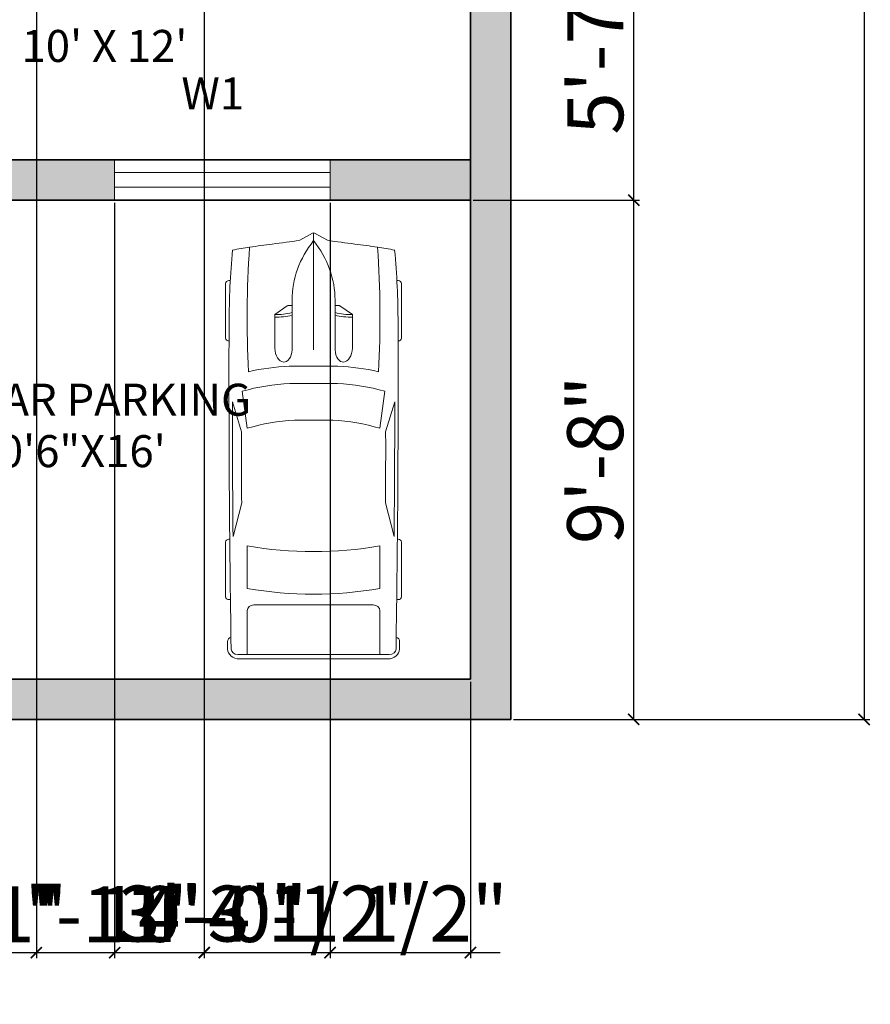
# Model space of a CAD drawing. Units: inches. Extents: x 1763 to 2368, y 1500 to 2097.
# Tile 13 of 24: x 2079 to 2269, y 1500 to 1720. Entities that reach past the tile are written whole.
import ezdxf

# ---------------------------------------------------------------- set-up
doc = ezdxf.new("R2010")
doc.units = ezdxf.units.IN
for name, color, linetype, lineweight in [('A-ANNO-DIMS', 2, 'Continuous', 18), ('A-ANNO-TEXT', 7, 'Continuous', 18), ('A-AREA-IDEN', 7, 'Continuous', 18), ('A-WALL', 7, 'Continuous', 35), ('A-WALL-PATT', 7, 'Continuous', 13), ('C-SITE-VEHC', 8, 'Continuous', 13), ('windows', 1, 'Continuous', 18)]:
    doc.layers.add(name, color=color, linetype=linetype, lineweight=lineweight)
doc.styles.get("Standard").update_dxf_attribs({"font": 'arial.ttf'})
doc.dimstyles.new('ISO-25', dxfattribs={"dimtxt": 12.5, "dimasz": 2.5, "dimexe": 1.25, "dimexo": 0.625, "dimtad": 1, "dimdec": 0, "dimlunit": 4, "dimtxsty": 'Standard', "dimblk": 'ARCHTICK', "dimcen": 2.5, "dimclrd": 3, "dimclrt": 4, "dimadec": 0, "dimazin": 0, "dimtfac": 1, "dimtdec": 0, "dimtmove": 0, "dimatfit": 3, "dimfxl": 1, "dimarcsym": 0})

# ---------------------------------------------------------------- blocks, each defined once
blk = doc.blocks.new('*U9')
for p, q in [((21.1, 37.41), (21.1, 36.83)), ((46.55, 38.89), (22.35, 38.89)), ((47.8, 37.39), (47.8, 37.41)), ((87.99, 31.87), (74.76, 35.92)), ((134.31, 35.6), (119.29, 31.78)), ((135.45, 37.07), (135.45, 37.41)), ((136.7, 38.89), (160.9, 38.89)), ((162.15, 37.41), (162.15, 36.77)), ((70.03, 31.54), (86.41, 29.35)), ((186.47, -33.5), (186.47, 33.5)), ((188.4, -32.76), (188.4, 32.76)), ((138.42, 29.35), (157.25, 29.35)), ((164.52, 26.39), (164.52, -26.39)), ((186.47, 29.35), (167.01, 29.35)), ((32.27, 11.63), (36.13, 17.17)), ((36.13, 17.17), (50.94, 17.17)), ((29.77, 9.51), (51.68, 9.51)), ((32.12, 9.51), (32.12, 11.15)), ((58.92, -10.77), (58.92, 10.77)), ((66.55, -10.53), (66.55, 10.53)), ((186.47, -10.53), (186.47, 10.53)), ((3.27, 6.13), (0.1, 0.41)), ((82.74, 8.5), (82.74, -8.5)), ((0, 0), (51.68, 0)), ((0.1, -0.41), (3.27, -6.13)), ((29.77, -9.51), (51.68, -9.51)), ((32.12, -9.51), (32.12, -11.15)), ((32.27, -11.63), (36.13, -17.17)), ((36.13, -17.17), (50.94, -17.17)), ((86.41, -29.35), (70.03, -31.54)), ((157.25, -29.35), (138.42, -29.35)), ((167.01, -29.35), (186.47, -29.35)), ((87.99, -31.87), (74.76, -35.92)), ((134.31, -35.6), (119.29, -31.78)), ((21.1, -37.41), (21.1, -36.83)), ((46.55, -38.89), (22.35, -38.89)), ((47.8, -37.39), (47.8, -37.41)), ((135.45, -37.07), (135.45, -37.41)), ((136.7, -38.89), (160.9, -38.89)), ((162.15, -37.41), (162.15, -36.77))]:
    blk.add_line(p, q)
for centre, major_axis, ratio, start_param, end_param in [((266.03, -27.52), (0, 313.31), 0.842304, 1.367076, 1.39176), ((41.19, -490.86), (0, 528.23), 0.842304, 0.00281, 0.075598), ((22.35, 37.41), (0, -1.48), 0.842304, 3.141593, 4.712389), ((64.48, -10555.62), (0, 10593.03), 0.842304, -0.013397, 0.002797), ((46.55, 37.41), (0, 1.48), 0.842304, -1.570796, 0), ((64.48, -10555.62), (0, -10591.55), 0.842304, 3.133765, 3.140441), ((136.7, 37.41), (0, -1.48), 0.842304, 3.141593, 4.712389), ((160.9, 37.41), (0, 1.48), 0.842304, -1.570796, 0), ((180.63, 35.84), (0, 2.22), 0.842304, -0.013017, 1.249894), ((64.48, -10556.36), (0, 10595.31), 0.842304, -0.013397, -0.013017), ((183.98, 33.5), (0, -2.96), 0.842304, 1.570796, 3.128196), ((183.98, 32.76), (0, -5.25), 0.842304, 1.570796, 3.128196), ((135.29, 5.39), (0, 81.77), 0.842304, 1.245306, 1.50788), ((95.79, -3666.35), (0, -3698.24), 0.842304, 3.134049, 3.144098), ((259.18, -27.52), (0, -305.3), 0.842304, 4.528606, 4.561838), ((37.47, -593.96), (0, -623.33), 0.842304, 3.096046, 3.200911), ((134.4, 5.39), (0, -89.78), 0.842304, 4.449482, 4.652344), ((149.6, 2.8), (0, -79.58), 0.842304, 4.372215, 4.640744), ((17.08, 0), (0, 147.02), 0.842304, 4.511394, 4.913384), ((35.91, 0), (0, 147.02), 0.842304, 4.511394, 4.913384), ((167.01, 26.39), (0, 2.96), 0.842304, 0, 1.570796), ((-204.49, 52.4), (0, -250.96), 0.842304, 1.385369, 1.434372), ((13.04, 17.01), (0, 27.42), 0.842304, 4.435146, 4.718221), ((14.2, 17.01), (0, 27.42), 0.842304, 4.435146, 4.718221), ((50.79, 13.34), (6.34, -0.36), 0.603834, -1.395552, 1.581315), ((29.77, -46.66), (0, 56.17), 0.842304, 0, 0.590319), ((32.75, 11.15), (0, 0.74), 0.842304, 0.879714, 1.570796), ((0.62, 0), (0, -0.74), 0.842304, 4.131459, 5.293319), ((29.77, 46.66), (0, 56.17), 0.842304, 2.551274, 3.141593), ((-204.49, -52.4), (0, 250.96), 0.842304, -1.434372, -1.385369), ((149.6, -2.8), (0, -79.58), 0.842304, -1.499151, -1.230623), ((32.75, -11.15), (0, -0.74), 0.842304, 4.712389, 5.403472), ((13.04, -17.01), (0, -27.42), 0.842304, 1.564964, 1.848039), ((14.2, -17.01), (0, -27.42), 0.842304, 1.564964, 1.848039), ((134.4, -5.39), (0, -89.78), 0.842304, -1.510751, -1.307889), ((135.29, -5.39), (0, -81.77), 0.842304, -1.50788, -1.245306), ((259.18, 27.52), (0, 305.3), 0.842304, 1.721348, 1.754579), ((266.03, 27.52), (0, 313.31), 0.842304, 1.749832, 1.774517), ((37.47, 593.96), (0, -623.33), 0.842304, -0.059319, 0.045547), ((167.01, -26.39), (0, -2.96), 0.842304, 4.712389, 6.283185), ((95.79, 3666.35), (0, -3698.24), 0.842304, -0.002505, 0.007544), ((183.98, -33.5), (0, 2.96), 0.842304, 3.15499, 4.712389), ((183.98, -32.76), (0, -5.25), 0.842304, 0.013397, 1.570796), ((41.19, 490.86), (0, -528.23), 0.842304, -0.075598, -0.00281), ((22.35, -37.41), (0, 1.48), 0.842304, 1.570796, 3.141593), ((64.48, 10555.62), (0, 10593.03), 0.842304, 3.138796, 3.15499), ((46.55, -37.41), (0, -1.48), 0.842304, 0, 1.570796), ((64.48, 10555.62), (0, -10591.55), 0.842304, 0.001152, 0.007828), ((136.7, -37.41), (0, -1.48), 0.842304, -1.570796, 0), ((160.9, -37.41), (0, 1.48), 0.842304, 3.141593, 4.712389), ((180.63, -35.84), (0, -2.22), 0.842304, -1.249894, 0.013017), ((64.48, 10556.36), (0, 10595.31), 0.842304, 3.15461, 3.15499)]:
    blk.add_ellipse(centre, major_axis=major_axis, ratio=ratio, start_param=start_param, end_param=end_param)
at = {"extrusion": (0, 0, -1)}
blk.add_ellipse((50.79, -13.34), major_axis=(6.34, 0.36), ratio=0.603834, start_param=-1.395552, end_param=1.581315, dxfattribs=at)
blk = doc.blocks.new('_ArchTick')
at = {"color": 0, "linetype": 'ByBlock', "const_width": 0.15}
blk.add_lwpolyline([(-0.5, -0.5), (0.5, 0.5)], dxfattribs=at)
blk = doc.blocks.new('*D22')
at = {"layer": 'A-ANNO-DIMS', "color": 0, "lineweight": -2, "transparency": 16777216}
for p, q in [((2189.72, 2043.27), (2269.32, 2043.27)), ((2268.07, 2043.27), (2268.07, 1563.27)), ((2189.72, 1563.27), (2269.32, 1563.27))]:
    blk.add_line(p, q, dxfattribs=at)
at = {"layer": 'Defpoints', "color": 0, "transparency": 16777216}
for p in [(2189.09, 2043.27), (2189.09, 1563.27), (2268.07, 1563.27)]:
    blk.add_point(p, dxfattribs=at)
at = {"layer": 'A-ANNO-DIMS', "color": 0, "lineweight": -2, "transparency": 16777216, "xscale": 2.5, "yscale": 2.5, "zscale": 2.5}
for p, rotation in [((2268.07, 2043.27), 90), ((2268.07, 1563.27), 270)]:
    blk.add_blockref('_ArchTick', p, dxfattribs=dict(at, rotation=rotation))
at = {"layer": 'A-ANNO-DIMS', "color": 0, "transparency": 16777216, "insert": (2261.06, 1803.27), "char_height": 12.5, "attachment_point": 5, "rotation": 90}
blk.add_mtext("40'", dxfattribs=at)
blk = doc.blocks.new('*D42')
at = {"layer": 'A-ANNO-DIMS', "color": 0, "lineweight": -2, "transparency": 16777216}
for p, q in [((2180.72, 1679.27), (2217.84, 1679.27)), ((2189.72, 1563.27), (2217.84, 1563.27))]:
    blk.add_line(p, q, dxfattribs=at)
at = {"layer": 'A-ANNO-DIMS', "color": 3, "lineweight": -2, "transparency": 16777216}
blk.add_line((2216.59, 1563.27), (2216.59, 1679.27), dxfattribs=at)
at = {"layer": 'Defpoints', "color": 0, "transparency": 16777216}
for p in [(2180.09, 1679.27), (2216.59, 1679.27), (2189.09, 1563.27)]:
    blk.add_point(p, dxfattribs=at)
at = {"layer": 'A-ANNO-DIMS', "color": 3, "lineweight": -2, "transparency": 16777216, "xscale": 2.5, "yscale": 2.5, "zscale": 2.5}
for p, rotation in [((2216.59, 1679.27), 90), ((2216.59, 1563.27), 270)]:
    blk.add_blockref('_ArchTick', p, dxfattribs=dict(at, rotation=rotation))
at = {"layer": 'A-ANNO-DIMS', "color": 4, "transparency": 16777216, "insert": (2209.58, 1621.27), "char_height": 12.5, "attachment_point": 5, "rotation": 90}
blk.add_mtext('9\'-8"', dxfattribs=at)
blk = doc.blocks.new('*D43')
at = {"layer": 'A-ANNO-DIMS', "color": 0, "lineweight": -2, "transparency": 16777216}
for p, q in [((2060.09, 1589.65), (2060.09, 1509.91)), ((2180.09, 1571.65), (2180.09, 1509.91))]:
    blk.add_line(p, q, dxfattribs=at)
at = {"layer": 'A-ANNO-DIMS', "color": 3, "lineweight": -2, "transparency": 16777216}
blk.add_line((2060.09, 1511.16), (2180.09, 1511.16), dxfattribs=at)
at = {"layer": 'Defpoints', "color": 0, "transparency": 16777216}
for p in [(2060.09, 1590.27), (2180.09, 1572.27), (2180.09, 1511.16)]:
    blk.add_point(p, dxfattribs=at)
at = {"layer": 'A-ANNO-DIMS', "color": 3, "lineweight": -2, "transparency": 16777216, "xscale": 2.5, "yscale": 2.5, "zscale": 2.5, "rotation": 180}
blk.add_blockref('_ArchTick', (2060.09, 1511.16), dxfattribs=at)
at = {"layer": 'A-ANNO-DIMS', "color": 3, "lineweight": -2, "transparency": 16777216, "xscale": 2.5, "yscale": 2.5, "zscale": 2.5}
blk.add_blockref('_ArchTick', (2180.09, 1511.16), dxfattribs=at)
at = {"layer": 'A-ANNO-DIMS', "color": 4, "transparency": 16777216, "insert": (2120.09, 1518.16), "char_height": 12.5, "attachment_point": 5}
blk.add_mtext('10\'-0"', dxfattribs=at)
blk = doc.blocks.new('*D52')
at = {"layer": 'A-ANNO-DIMS', "color": 0, "lineweight": -2, "transparency": 16777216}
for p, q in [((2189.72, 1746.22), (2217.84, 1746.22)), ((2180.72, 1679.27), (2217.84, 1679.27))]:
    blk.add_line(p, q, dxfattribs=at)
at = {"layer": 'A-ANNO-DIMS', "color": 3, "lineweight": -2, "transparency": 16777216}
blk.add_line((2216.59, 1679.27), (2216.59, 1746.22), dxfattribs=at)
at = {"layer": 'Defpoints', "color": 0, "transparency": 16777216}
for p in [(2189.09, 1746.22), (2216.59, 1746.22), (2180.09, 1679.27)]:
    blk.add_point(p, dxfattribs=at)
at = {"layer": 'A-ANNO-DIMS', "color": 3, "lineweight": -2, "transparency": 16777216, "xscale": 2.5, "yscale": 2.5, "zscale": 2.5}
for p, rotation in [((2216.59, 1746.22), 90), ((2216.59, 1679.27), 270)]:
    blk.add_blockref('_ArchTick', p, dxfattribs=dict(at, rotation=rotation))
at = {"layer": 'A-ANNO-DIMS', "color": 4, "transparency": 16777216, "insert": (2209.61, 1712.75), "char_height": 12.5, "attachment_point": 5, "rotation": 90}
blk.add_mtext('5\'-7"', dxfattribs=at)
blk = doc.blocks.new('*D59')
at = {"layer": 'A-ANNO-DIMS', "color": 0, "lineweight": -2, "transparency": 16777216}
for p, q in [((2019.39, 1625.65), (2019.39, 1509.91)), ((2042.48, 1625.65), (2042.48, 1509.91))]:
    blk.add_line(p, q, dxfattribs=at)
at = {"layer": 'A-ANNO-DIMS', "color": 3, "lineweight": -2, "transparency": 16777216}
for p, q in [((2019.39, 1511.16), (2042.48, 1511.16)), ((2042.48, 1511.16), (2088, 1511.16))]:
    blk.add_line(p, q, dxfattribs=at)
at = {"layer": 'Defpoints', "color": 0, "transparency": 16777216}
for p in [(2019.39, 1626.27), (2042.48, 1626.27), (2042.48, 1511.16)]:
    blk.add_point(p, dxfattribs=at)
at = {"layer": 'A-ANNO-DIMS', "color": 3, "lineweight": -2, "transparency": 16777216, "xscale": 2.5, "yscale": 2.5, "zscale": 2.5, "rotation": 180}
blk.add_blockref('_ArchTick', (2019.39, 1511.16), dxfattribs=at)
at = {"layer": 'A-ANNO-DIMS', "color": 3, "lineweight": -2, "transparency": 16777216, "xscale": 2.5, "yscale": 2.5, "zscale": 2.5}
blk.add_blockref('_ArchTick', (2042.48, 1511.16), dxfattribs=at)
at = {"layer": 'A-ANNO-DIMS', "color": 4, "transparency": 16777216, "insert": (2066.49, 1518.06), "char_height": 12.5, "attachment_point": 5}
blk.add_mtext('1\'-11"', dxfattribs=at)
blk = doc.blocks.new('*D60')
at = {"layer": 'A-ANNO-DIMS', "color": 0, "lineweight": -2, "transparency": 16777216}
for p, q in [((2060.09, 1678.65), (2060.09, 1509.91)), ((2100.58, 1678.65), (2100.58, 1509.91))]:
    blk.add_line(p, q, dxfattribs=at)
at = {"layer": 'A-ANNO-DIMS', "color": 3, "lineweight": -2, "transparency": 16777216}
for p, q in [((2060.09, 1511.16), (2100.58, 1511.16)), ((2100.58, 1511.16), (2166.67, 1511.16))]:
    blk.add_line(p, q, dxfattribs=at)
at = {"layer": 'Defpoints', "color": 0, "transparency": 16777216}
for p in [(2060.09, 1679.27), (2100.58, 1679.27), (2100.58, 1511.16)]:
    blk.add_point(p, dxfattribs=at)
at = {"layer": 'A-ANNO-DIMS', "color": 3, "lineweight": -2, "transparency": 16777216, "xscale": 2.5, "yscale": 2.5, "zscale": 2.5, "rotation": 180}
blk.add_blockref('_ArchTick', (2060.09, 1511.16), dxfattribs=at)
at = {"layer": 'A-ANNO-DIMS', "color": 3, "lineweight": -2, "transparency": 16777216, "xscale": 2.5, "yscale": 2.5, "zscale": 2.5}
blk.add_blockref('_ArchTick', (2100.58, 1511.16), dxfattribs=at)
at = {"layer": 'A-ANNO-DIMS', "color": 4, "transparency": 16777216, "insert": (2134.88, 1518.25), "char_height": 12.5, "attachment_point": 5}
blk.add_mtext('3\'-4 1/2"', dxfattribs=at)
blk = doc.blocks.new('*D61')
at = {"layer": 'A-ANNO-DIMS', "color": 0, "lineweight": -2, "transparency": 16777216}
for p, q in [((2100.58, 1678.65), (2100.58, 1509.91)), ((2148.74, 1678.65), (2148.74, 1509.91))]:
    blk.add_line(p, q, dxfattribs=at)
at = {"layer": 'A-ANNO-DIMS', "color": 3, "lineweight": -2, "transparency": 16777216}
blk.add_line((2100.58, 1511.16), (2148.74, 1511.16), dxfattribs=at)
at = {"layer": 'Defpoints', "color": 0, "transparency": 16777216}
for p in [(2100.58, 1679.27), (2148.74, 1679.27), (2148.74, 1511.16)]:
    blk.add_point(p, dxfattribs=at)
at = {"layer": 'A-ANNO-DIMS', "color": 3, "lineweight": -2, "transparency": 16777216, "xscale": 2.5, "yscale": 2.5, "zscale": 2.5, "rotation": 180}
blk.add_blockref('_ArchTick', (2100.58, 1511.16), dxfattribs=at)
at = {"layer": 'A-ANNO-DIMS', "color": 3, "lineweight": -2, "transparency": 16777216, "xscale": 2.5, "yscale": 2.5, "zscale": 2.5}
blk.add_blockref('_ArchTick', (2148.74, 1511.16), dxfattribs=at)
at = {"layer": 'A-ANNO-DIMS', "color": 4, "transparency": 16777216, "insert": (2124.66, 1518.16), "char_height": 12.5, "attachment_point": 5}
blk.add_mtext('4\'-0"', dxfattribs=at)
blk = doc.blocks.new('*D62')
at = {"layer": 'A-ANNO-DIMS', "color": 0, "lineweight": -2, "transparency": 16777216}
for p, q in [((2083.09, 1980.65), (2083.09, 1509.91)), ((2120.61, 1980.65), (2120.61, 1509.91))]:
    blk.add_line(p, q, dxfattribs=at)
at = {"layer": 'A-ANNO-DIMS', "color": 3, "lineweight": -2, "transparency": 16777216}
for p, q in [((2083.09, 1511.16), (2120.61, 1511.16)), ((2120.61, 1511.16), (2186.71, 1511.16))]:
    blk.add_line(p, q, dxfattribs=at)
at = {"layer": 'Defpoints', "color": 0, "transparency": 16777216}
for p in [(2083.09, 1981.27), (2120.61, 1981.27), (2120.61, 1511.16)]:
    blk.add_point(p, dxfattribs=at)
at = {"layer": 'A-ANNO-DIMS', "color": 3, "lineweight": -2, "transparency": 16777216, "xscale": 2.5, "yscale": 2.5, "zscale": 2.5, "rotation": 180}
blk.add_blockref('_ArchTick', (2083.09, 1511.16), dxfattribs=at)
at = {"layer": 'A-ANNO-DIMS', "color": 3, "lineweight": -2, "transparency": 16777216, "xscale": 2.5, "yscale": 2.5, "zscale": 2.5}
blk.add_blockref('_ArchTick', (2120.61, 1511.16), dxfattribs=at)
at = {"layer": 'A-ANNO-DIMS', "color": 4, "transparency": 16777216, "insert": (2154.91, 1518.25), "char_height": 12.5, "attachment_point": 5}
blk.add_mtext('3\'-1 1/2"', dxfattribs=at)
blk = doc.blocks.new('*D71')
at = {"layer": 'A-ANNO-DIMS', "color": 0, "lineweight": -2, "transparency": 16777216}
for p, q in [((2049.69, 1879.65), (2049.69, 1509.91)), ((2072.78, 1879.65), (2072.78, 1509.91))]:
    blk.add_line(p, q, dxfattribs=at)
at = {"layer": 'A-ANNO-DIMS', "color": 3, "lineweight": -2, "transparency": 16777216}
for p, q in [((2049.69, 1511.16), (2072.78, 1511.16)), ((2072.78, 1511.16), (2118.3, 1511.16))]:
    blk.add_line(p, q, dxfattribs=at)
at = {"layer": 'Defpoints', "color": 0, "transparency": 16777216}
for p in [(2049.69, 1880.27), (2072.78, 1880.27), (2072.78, 1511.16)]:
    blk.add_point(p, dxfattribs=at)
at = {"layer": 'A-ANNO-DIMS', "color": 3, "lineweight": -2, "transparency": 16777216, "xscale": 2.5, "yscale": 2.5, "zscale": 2.5, "rotation": 180}
blk.add_blockref('_ArchTick', (2049.69, 1511.16), dxfattribs=at)
at = {"layer": 'A-ANNO-DIMS', "color": 3, "lineweight": -2, "transparency": 16777216, "xscale": 2.5, "yscale": 2.5, "zscale": 2.5}
blk.add_blockref('_ArchTick', (2072.78, 1511.16), dxfattribs=at)
at = {"layer": 'A-ANNO-DIMS', "color": 4, "transparency": 16777216, "insert": (2096.79, 1518.06), "char_height": 12.5, "attachment_point": 5}
blk.add_mtext('1\'-11"', dxfattribs=at)
blk = doc.blocks.new('*D83')
at = {"layer": 'A-ANNO-DIMS', "color": 0, "lineweight": -2, "transparency": 16777216}
for p, q in [((2005.2, 1589.65), (2005.2, 1509.91)), ((2040.27, 1589.65), (2040.27, 1509.91))]:
    blk.add_line(p, q, dxfattribs=at)
at = {"layer": 'A-ANNO-DIMS', "color": 3, "lineweight": -2, "transparency": 16777216}
for p, q in [((2005.2, 1511.16), (2040.27, 1511.16)), ((2040.27, 1511.16), (2087.17, 1511.16))]:
    blk.add_line(p, q, dxfattribs=at)
at = {"layer": 'Defpoints', "color": 0, "transparency": 16777216}
for p in [(2005.2, 1590.27), (2040.27, 1590.27), (2040.27, 1511.16)]:
    blk.add_point(p, dxfattribs=at)
at = {"layer": 'A-ANNO-DIMS', "color": 3, "lineweight": -2, "transparency": 16777216, "xscale": 2.5, "yscale": 2.5, "zscale": 2.5, "rotation": 180}
blk.add_blockref('_ArchTick', (2005.2, 1511.16), dxfattribs=at)
at = {"layer": 'A-ANNO-DIMS', "color": 3, "lineweight": -2, "transparency": 16777216, "xscale": 2.5, "yscale": 2.5, "zscale": 2.5}
blk.add_blockref('_ArchTick', (2040.27, 1511.16), dxfattribs=at)
at = {"layer": 'A-ANNO-DIMS', "color": 4, "transparency": 16777216, "insert": (2064.97, 1518.06), "char_height": 12.5, "attachment_point": 5}
blk.add_mtext('2\'-11"', dxfattribs=at)

msp = doc.modelspace()

# ---------------------------------------------------------------- hatches: boundary and pattern name
at = {"layer": 'A-WALL-PATT'}
h = msp.add_hatch(color=256, dxfattribs=at)
h.dxf.hatch_style = 1
h.paths.add_polyline_path([(1838.09, 2034.27), (1838.09, 2043.27), (1829.09, 2043.27), (1829.09, 1953.39), (1838.09, 1953.39)])
h.paths.add_polyline_path([(1838.09, 1913.1), (1829.09, 1913.1), (1829.09, 1862.2), (1838.09, 1862.2)])
h.paths.add_polyline_path([(1838.09, 1825.59), (1829.09, 1825.59), (1829.09, 1738.64), (1838.09, 1738.64)])
h.paths.add_polyline_path([(1895.59, 1885.27), (1838.09, 1885.27), (1838.09, 1880.27), (1895.59, 1880.27)])
h.paths.add_polyline_path([(1857.39, 1784.27), (1838.09, 1784.27), (1838.09, 1779.27), (1857.39, 1779.27)])
h.paths.add_polyline_path([(1958.09, 1981.27), (1971.46, 1981.27), (1971.46, 1986.27), (1968.57, 1986.27), (1958.09, 1986.27), (1953.09, 1986.27), (1927.39, 1986.27), (1927.39, 1981.27), (1953.09, 1981.27), (1953.09, 1885.27), (1932.01, 1885.27), (1932.01, 1880.27), (1959.13, 1880.27), (1959.13, 1883.74), (1959.13, 1885.27), (1958.09, 1885.27)])
h.paths.add_polyline_path([(2018.09, 1981.27), (2031.02, 1981.27), (2031.02, 1986.27), (2018.09, 1986.27), (2013.09, 1986.27), (2001.23, 1986.27), (2001.23, 1981.27), (2013.09, 1981.27), (2013.09, 1885.27), (1982.18, 1885.27, -0.016629), (1982.23, 1883.74), (1982.23, 1880.27), (2049.69, 1880.27), (2049.69, 1883.74, -0.016629), (2049.74, 1885.27), (2018.09, 1885.27)])
h.paths.add_polyline_path([(2083.09, 1981.27), (2120.61, 1981.27), (2120.61, 1986.27), (2083.09, 1986.27), (2078.09, 1986.27), (2063.14, 1986.27), (2063.14, 1981.27), (2078.09, 1981.27), (2078.09, 1885.27), (2072.78, 1885.27), (2072.78, 1883.74), (2072.78, 1880.27), (2078.09, 1880.27), (2078.09, 1866.87), (2081.56, 1866.87, -0.016629), (2083.09, 1866.82)])
h.paths.add_polyline_path([(1871.68, 1635.27), (1838.09, 1635.27), (1838.09, 1626.27), (1871.68, 1626.27)], flags=17)
h.paths.add_polyline_path([(2100.58, 1688.27), (2060.09, 1688.27), (2060.09, 1679.27), (2100.58, 1679.27)], flags=17)
h.paths.add_polyline_path([(2180.09, 1688.27), (2148.74, 1688.27), (2148.74, 1679.27), (2180.09, 1679.27)], flags=17)
h.paths.add_polyline_path([(2189.09, 1746.22), (2180.09, 1746.22), (2180.09, 1743.42), (2180.12, 1743.42), (2180.12, 1726.72), (2180.09, 1572.27), (2034.91, 1572.27), (2034.91, 1565.6), (2034.91, 1563.27), (2189.09, 1563.27)])
h.paths.add_polyline_path([(2060.09, 1802.35, -0.016629), (2058.56, 1802.3), (2055.09, 1802.3), (2055.09, 1635.27), (2042.48, 1635.27), (2042.48, 1629.74), (2042.48, 1626.27), (2055.09, 1626.27), (2055.09, 1599.27), (2040.27, 1599.27), (2040.27, 1590.27), (2060.09, 1590.27)])
h.paths.add_polyline_path([(2019.39, 1629.74, -0.060569), (2020.06, 1635.27), (1995.09, 1635.27), (1990.09, 1635.27), (1927.07, 1635.27), (1927.07, 1626.27), (1990.09, 1626.27), (1990.09, 1590.27), (1995.09, 1590.27), (2005.2, 1590.27), (2005.2, 1599.27), (1995.09, 1599.27), (1995.09, 1626.27), (2019.39, 1626.27)])
edge = h.paths.add_edge_path()
edge.add_line((2180.09, 1837.27), (2167.2, 1837.27))
edge.add_spline(control_points=[(2167.2, 1837.27), (2167.19, 1837.27), (2167.18, 1837.27), (2167.18, 1837.27)], knot_values=[168.955493, 168.955493, 168.955493, 168.955493, 169.065871, 169.065871, 169.065871, 169.065871], degree=3, periodic=0)
edge.add_spline(control_points=[(2167.18, 1837.27), (2166.56, 1837.38), (2166.33, 1846.16), (2165.71, 1846.24)], knot_values=[159.864705, 159.864705, 159.864705, 159.864705, 168.955493, 168.955493, 168.955493, 168.955493], degree=3, periodic=0)
edge.add_line((2167.12, 1837.27), (2163.16, 1837.27))
edge.add_spline(control_points=[(2163.16, 1837.27), (2163.16, 1837.27), (2163.16, 1837.27), (2163.15, 1837.27)], knot_values=[150.537172, 150.537172, 150.537172, 150.537172, 150.553797, 150.553797, 150.553797, 150.553797], degree=3, periodic=0)
edge.add_spline(control_points=[(2163.15, 1837.27), (2162.29, 1837.29), (2161.59, 1846.23), (2160.88, 1846.24)], knot_values=[141.293426, 141.293426, 141.293426, 141.293426, 150.537172, 150.537172, 150.537172, 150.537172], degree=3, periodic=0)
edge.add_line((2163.08, 1837.27), (2158.7, 1837.27))
edge.add_spline(control_points=[(2158.7, 1837.27), (2158.7, 1837.27), (2158.7, 1837.27), (2158.7, 1837.27)], knot_values=[132.033544, 132.033544, 132.033544, 132.033544, 132.049151, 132.049151, 132.049151, 132.049151], degree=3, periodic=0)
edge.add_spline(control_points=[(2158.7, 1837.27), (2157.97, 1837.29), (2157.26, 1846.23), (2156.39, 1846.24)], knot_values=[122.786021, 122.786021, 122.786021, 122.786021, 132.033544, 132.033544, 132.033544, 132.033544], degree=3, periodic=0)
edge.add_line((2158.63, 1837.27), (2153.84, 1837.27))
edge.add_spline(control_points=[(2153.84, 1837.27), (2153.83, 1837.27), (2153.82, 1837.27), (2153.82, 1837.27)], knot_values=[113.451585, 113.451585, 113.451585, 113.451585, 113.562103, 113.562103, 113.562103, 113.562103], degree=3, periodic=0)
edge.add_spline(control_points=[(2153.82, 1837.27), (2153.17, 1837.38), (2152.88, 1846.19), (2152.4, 1846.24)], knot_values=[0, 0, 0, 0, 9.081854, 9.081854, 9.081854, 9.081854], degree=3, periodic=0)
edge.add_line((2153.76, 1837.27), (2150.39, 1837.27))
edge.add_spline(control_points=[(2150.39, 1837.27), (2150.38, 1837.27), (2150.37, 1837.27), (2150.36, 1837.27)], knot_values=[95.069382, 95.069382, 95.069382, 95.069382, 95.17519, 95.17519, 95.17519, 95.17519], degree=3, periodic=0)
edge.add_spline(control_points=[(2150.36, 1837.27), (2149.49, 1837.37), (2148.42, 1846.19), (2147.59, 1846.24)], knot_values=[85.824599, 85.824599, 85.824599, 85.824599, 95.069382, 95.069382, 95.069382, 95.069382], degree=3, periodic=0)
edge.add_line((2150.29, 1837.27), (2145.43, 1837.27))
edge.add_spline(control_points=[(2145.43, 1837.27), (2145.43, 1837.27), (2145.42, 1837.27), (2145.42, 1837.27)], knot_values=[76.505559, 76.505559, 76.505559, 76.505559, 76.547811, 76.547811, 76.547811, 76.547811], degree=3, periodic=0)
edge.add_spline(control_points=[(2145.42, 1837.27), (2144.68, 1837.31), (2143.8, 1846.19), (2142.95, 1846.24)], knot_values=[67.23945, 67.23945, 67.23945, 67.23945, 76.505559, 76.505559, 76.505559, 76.505559], degree=3, periodic=0)
edge.add_line((2145.35, 1837.27), (2134.57, 1837.27))
edge.add_spline(control_points=[(2134.57, 1837.27), (2134.57, 1837.27), (2134.56, 1837.27), (2134.56, 1837.27)], knot_values=[39.001463, 39.001463, 39.001463, 39.001463, 39.045107, 39.045107, 39.045107, 39.045107], degree=3, periodic=0)
edge.add_spline(control_points=[(2134.56, 1837.27), (2133.87, 1837.31), (2133.4, 1845.85), (2132.33, 1846.24)], knot_values=[29.79778, 29.79778, 29.79778, 29.79778, 39.001463, 39.001463, 39.001463, 39.001463], degree=3, periodic=0)
edge.add_line((2134.5, 1837.27), (2128.08, 1837.27))
edge.add_spline(control_points=[(2128.08, 1837.27), (2128.03, 1837.26), (2127.98, 1837.26), (2127.93, 1837.27)], knot_values=[19.482067, 19.482067, 19.482067, 19.482067, 19.869396, 19.869396, 19.869396, 19.869396], degree=3, periodic=0)
edge.add_spline(control_points=[(2125.01, 1846.24), (2126.16, 1844.66), (2126.82, 1837.57), (2127.93, 1837.27)], knot_values=[10.389805, 10.389805, 10.389805, 10.389805, 19.482067, 19.482067, 19.482067, 19.482067], degree=3, periodic=0)
edge.add_line((2127.93, 1837.27), (2083.09, 1837.27))
edge.add_line((2083.09, 1837.27), (2083.09, 1843.77))
edge.add_line((2083.09, 1843.77), (2081.56, 1843.77))
edge.add_line((2081.56, 1843.77), (2078.09, 1843.77))
edge.add_line((2078.09, 1843.77), (2078.09, 1837.27))
edge.add_line((2078.09, 1837.27), (2055.09, 1837.27))
edge.add_line((2055.09, 1837.27), (2055.09, 1825.4))
edge.add_line((2055.09, 1825.4), (2058.56, 1825.4))
edge.add_line((2058.56, 1825.4), (2060.09, 1825.4))
edge.add_line((2060.09, 1825.4), (2060.09, 1832.27))
edge.add_line((2060.09, 1832.27), (2122.44, 1832.27))
edge.add_spline(control_points=[(2122.44, 1832.27), (2122.73, 1832.58), (2123.01, 1832.62), (2123.28, 1832.27)], knot_values=[5.972033, 5.972033, 5.972033, 5.972033, 8.057258, 8.057258, 8.057258, 8.057258], degree=3, periodic=0)
edge.add_line((2123.28, 1832.27), (2137.95, 1832.27))
edge.add_spline(control_points=[(2137.95, 1832.27), (2137.96, 1832.27), (2137.97, 1832.27), (2137.98, 1832.27)], knot_values=[53.926862, 53.926862, 53.926862, 53.926862, 54.030075, 54.030075, 54.030075, 54.030075], degree=3, periodic=0)
edge.add_spline(control_points=[(2139.72, 1825.02), (2139.28, 1825.06), (2138.67, 1832.18), (2137.98, 1832.27)], knot_values=[54.030075, 54.030075, 54.030075, 54.030075, 61.445194, 61.445194, 61.445194, 61.445194], degree=3, periodic=0)
edge.add_line((2138.05, 1832.27), (2140.96, 1832.27))
edge.add_spline(control_points=[(2140.96, 1832.27), (2140.97, 1832.27), (2140.98, 1832.27), (2140.99, 1832.27)], knot_values=[68.854182, 68.854182, 68.854182, 68.854182, 68.971237, 68.971237, 68.971237, 68.971237], degree=3, periodic=0)
edge.add_spline(control_points=[(2143.19, 1825.02), (2142.44, 1825.07), (2141.56, 1832.16), (2140.99, 1832.27)], knot_values=[68.971237, 68.971237, 68.971237, 68.971237, 76.444911, 76.444911, 76.444911, 76.444911], degree=3, periodic=0)
edge.add_line((2141.04, 1832.27), (2145.43, 1832.27))
edge.add_spline(control_points=[(2145.43, 1832.27), (2145.44, 1832.27), (2145.45, 1832.27), (2145.46, 1832.27)], knot_values=[84.039047, 84.039047, 84.039047, 84.039047, 84.124041, 84.124041, 84.124041, 84.124041], degree=3, periodic=0)
edge.add_spline(control_points=[(2148.11, 1825.02), (2147.34, 1825.02), (2146.3, 1832.19), (2145.46, 1832.27)], knot_values=[84.124041, 84.124041, 84.124041, 84.124041, 91.773891, 91.773891, 91.773891, 91.773891], degree=3, periodic=0)
edge.add_line((2145.54, 1832.27), (2150.39, 1832.27))
edge.add_spline(control_points=[(2150.39, 1832.27), (2150.42, 1832.28), (2150.45, 1832.28), (2150.47, 1832.27)], knot_values=[99.381577, 99.381577, 99.381577, 99.381577, 99.573457, 99.573457, 99.573457, 99.573457], degree=3, periodic=0)
edge.add_spline(control_points=[(2153.97, 1825.02), (2153.09, 1825.28), (2151.53, 1832.1), (2150.47, 1832.27)], knot_values=[99.573457, 99.573457, 99.573457, 99.573457, 107.218357, 107.218357, 107.218357, 107.218357], degree=3, periodic=0)
edge.add_line((2150.57, 1832.27), (2155.6, 1832.27))
edge.add_spline(control_points=[(2155.6, 1832.27), (2155.6, 1832.27), (2155.61, 1832.27), (2155.62, 1832.27)], knot_values=[114.933058, 114.933058, 114.933058, 114.933058, 115.013624, 115.013624, 115.013624, 115.013624], degree=3, periodic=0)
edge.add_spline(control_points=[(2158.28, 1825.02), (2157.4, 1825.07), (2156.25, 1832.2), (2155.62, 1832.27)], knot_values=[115.013624, 115.013624, 115.013624, 115.013624, 122.616269, 122.616269, 122.616269, 122.616269], degree=3, periodic=0)
edge.add_line((2155.68, 1832.27), (2165.19, 1832.27))
edge.add_spline(control_points=[(2165.19, 1832.27), (2165.2, 1832.27), (2165.2, 1832.27), (2165.2, 1832.27)], knot_values=[145.488477, 145.488477, 145.488477, 145.488477, 145.516379, 145.516379, 145.516379, 145.516379], degree=3, periodic=0)
edge.add_spline(control_points=[(2167.45, 1825.02), (2166.96, 1825.02), (2166.06, 1832.25), (2165.2, 1832.27)], knot_values=[145.516379, 145.516379, 145.516379, 145.516379, 153.105469, 153.105469, 153.105469, 153.105469], degree=3, periodic=0)
edge.add_line((2165.29, 1832.27), (2168.93, 1832.27))
edge.add_spline(control_points=[(2168.93, 1832.27), (2168.98, 1832.29), (2169.04, 1832.29), (2169.1, 1832.27)], knot_values=[160.517439, 160.517439, 160.517439, 160.517439, 160.939723, 160.939723, 160.939723, 160.939723], degree=3, periodic=0)
edge.add_spline(control_points=[(2171.09, 1828.64), (2170.35, 1830.37), (2169.62, 1832.09), (2169.1, 1832.27)], knot_values=[160.939723, 160.939723, 160.939723, 160.939723, 164.738835, 164.738835, 164.738835, 164.738835], degree=3, periodic=0)
edge.add_line((2169.1, 1832.27), (2180.09, 1832.27))
edge.add_line((2180.09, 1832.27), (2180.09, 1837.27))
h.paths.add_polyline_path([(2189.09, 1885.52), (2180.09, 1885.52), (2180.09, 1813.32), (2180.12, 1813.32), (2180.12, 1796.62), (2180.12, 1795.26), (2189.09, 1795.26)])
h.paths.add_polyline_path([(2180.09, 1986.27), (2166.28, 1986.27), (2166.28, 1981.27), (2180.09, 1981.27)])
h.paths.add_polyline_path([(2189.09, 2043.27), (2180.09, 2043.27), (2180.09, 2034.27), (2180.09, 1934.11), (2189.09, 1934.11)])
h.paths.add_polyline_path([(1838.09, 1681.59), (1829.09, 1681.59), (1829.09, 1563.27), (2003.86, 1563.27), (2003.86, 1565.6), (2003.86, 1572.27), (1838.09, 1572.27)])

# ---------------------------------------------------------------- linework, layer by layer
at = {"layer": 'A-WALL'}
for p, q in [((2180.09, 2034.27), (2180.09, 1572.27)), ((2060.09, 1688.27), (2180.09, 1688.27)), ((2060.09, 1679.27), (2180.09, 1679.27)), ((2180.09, 1572.27), (2034.23, 1572.27))]:
    msp.add_line(p, q, dxfattribs=at)
msp.add_lwpolyline([(2003.86, 1563.27), (1829.09, 1563.27), (1829.09, 2043.27), (2189.09, 2043.27), (2189.09, 1563.27), (2034.91, 1563.27)], dxfattribs=at)
at = {"layer": 'windows'}
for p, q in [((2100.58, 1688.27), (2100.58, 1679.27)), ((2148.74, 1688.27), (2100.58, 1688.27)), ((2148.74, 1679.27), (2148.74, 1688.27)), ((2100.58, 1685.44), (2148.74, 1685.44)), ((2100.58, 1682.19), (2148.74, 1682.19)), ((2100.58, 1679.27), (2148.74, 1679.27))]:
    msp.add_line(p, q, dxfattribs=at)

# ---------------------------------------------------------------- block references
at = {"layer": 'C-SITE-VEHC', "xscale": 0.5052682773730944, "yscale": 0.5052682773730944, "zscale": 0.5052682773730944, "rotation": 270}
msp.add_blockref('*U9', (2145.04, 1671.96), dxfattribs=at)

# ---------------------------------------------------------------- texts
at = {"layer": 'A-ANNO-TEXT'}
msp.add_text('W1', height=7.155, dxfattribs=at).set_placement((2115.51, 1699.53))
at = {"layer": 'A-AREA-IDEN'}
for s, height, p in [("10' X 12'", 7.155, (2079.79, 1710.15)), ('CAR PARKING', 7.1545, (2069.29, 1631.11)), ('10\'6"X16\'', 7.155, (2069.29, 1619.62))]:
    msp.add_text(s, height=height, dxfattribs=at).set_placement(p)

# ---------------------------------------------------------------- dimensions: what is measured, and where the dimension line sits
at = {"layer": 'A-ANNO-DIMS'}
for base, p1, p2, override, picture, middle in [((2268.07, 1563.27), (2189.09, 2043.27), (2189.09, 1563.27), {"dimclrd": 0, "dimclre": 0, "dimclrt": 0}, '*D22', (2261.06, 1803.27)), ((2216.5918, 1746.2191), (2180.0918, 1679.2727), (2189.0918, 1746.2191), {"dimdec": 1, "dimlfac": 1, "dimrnd": 0, "dimzin": 1, "dimdsep": 46, "dimlunit": 4, "dimfrac": 2}, '*D52', (2209.6102, 1712.7459)), ((2216.59, 1679.27), (2189.09, 1563.27), (2180.09, 1679.27), {"dimdec": 1, "dimlfac": 1, "dimrnd": 0, "dimzin": 1, "dimdsep": 46, "dimlunit": 4, "dimfrac": 2}, '*D42', (2209.58, 1621.27))]:
    dim = msp.add_linear_dim(base=base, p1=p1, p2=p2, angle=90, dimstyle='ISO-25', override=override, dxfattribs=at)
    dim.commit()
    dim.dimension.update_dxf_attribs({"geometry": picture, "text_midpoint": middle})
for base, p1, p2, picture, middle in [((2120.61, 1511.16), (2083.09, 1981.27), (2120.61, 1981.27), '*D62', (2154.91, 1518.25)), ((2072.78, 1511.16), (2049.69, 1880.27), (2072.78, 1880.27), '*D71', (2096.79, 1518.06)), ((2100.58, 1511.16), (2060.09, 1679.27), (2100.58, 1679.27), '*D60', (2134.88, 1518.25)), ((2148.74, 1511.16), (2100.58, 1679.27), (2148.74, 1679.27), '*D61', (2124.66, 1518.16)), ((2042.48, 1511.16), (2019.39, 1626.27), (2042.48, 1626.27), '*D59', (2066.49, 1518.06)), ((2040.27, 1511.16), (2005.2, 1590.27), (2040.27, 1590.27), '*D83', (2064.97, 1518.06)), ((2180.09, 1511.16), (2060.09, 1590.27), (2180.09, 1572.27), '*D43', (2120.09, 1518.16))]:
    dim = msp.add_linear_dim(base=base, p1=p1, p2=p2, dimstyle='ISO-25', override={"dimdec": 1, "dimlfac": 1, "dimrnd": 0, "dimzin": 1, "dimdsep": 46, "dimlunit": 4, "dimfrac": 2}, dxfattribs=at)
    dim.commit()
    dim.dimension.update_dxf_attribs({"geometry": picture, "text_midpoint": middle})

doc.saveas('drawing.dxf')
